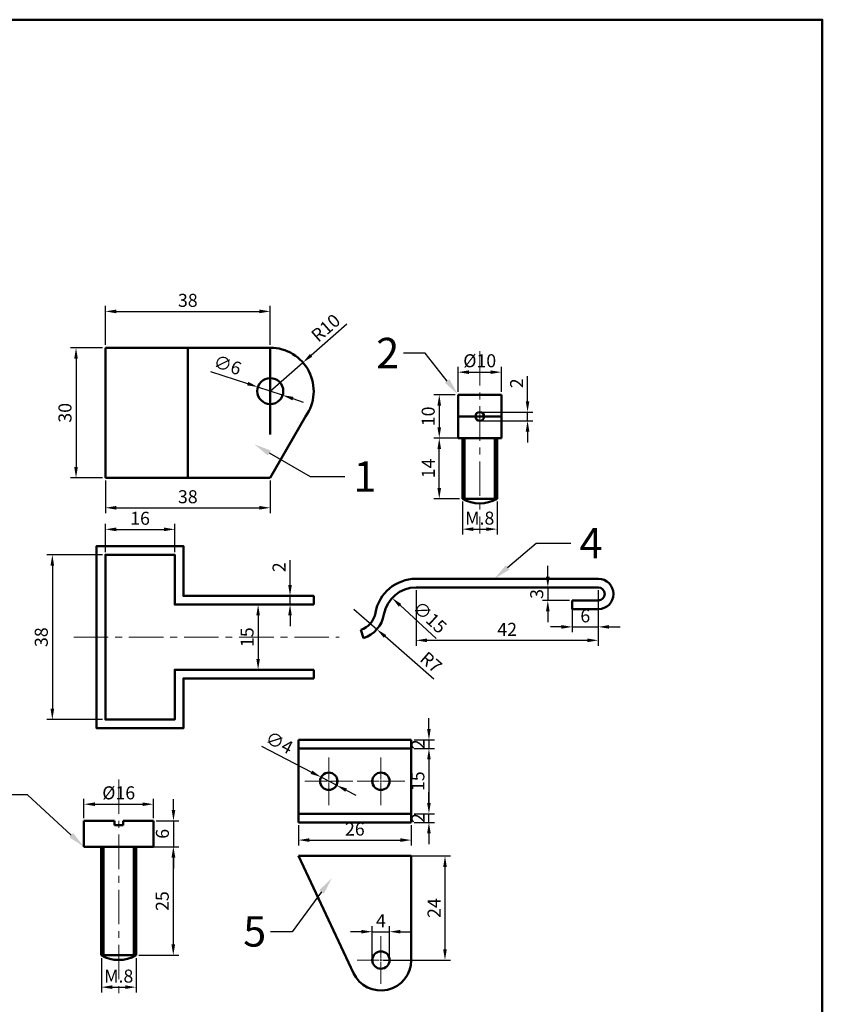
# Model space of a CAD drawing. Units: millimetres. Extents: x 77 to 718, y -35 to 313.
# Tile 7 of 7: x 533 to 718, y 86 to 313. Entities that reach past the tile are written whole.
import ezdxf
from ezdxf import colors
from ezdxf.entities.mleader import LeaderData, LeaderLine
from ezdxf.math import Vec2, Vec3

# ---------------------------------------------------------------- set-up
doc = ezdxf.new("R2010")
doc.units = ezdxf.units.MM
doc.header["$LTSCALE"] = 0.5
doc.linetypes.add('CENTER', pattern=[50.8, 31.75, -6.35, 6.35, -6.35])
for name, color, linetype, lineweight in [('M-CNTR', 1, 'CENTER', 18), ('M-DIMS', 2, 'Continuous', 25), ('M-OUTL', 7, 'Continuous', 50), ('M-TEXT', 3, 'Continuous', 25)]:
    doc.layers.add(name, color=color, linetype=linetype, lineweight=lineweight)
doc.styles.get("Standard").update_dxf_attribs({"font": 'arial.ttf'})
doc.dimstyles.new('ISO-25', dxfattribs={"dimtxt": 3, "dimasz": 2.5, "dimexe": 1.25, "dimexo": 0.625, "dimtad": 1, "dimtxsty": 'Standard', "dimcen": 2.5, "dimadec": 0, "dimazin": 0, "dimtfac": 1, "dimtmove": 0, "dimatfit": 3, "dimfxl": 1, "dimarcsym": 0})

# ---------------------------------------------------------------- blocks, each defined once
blk = doc.blocks.new('*D93')
at = {"layer": 'Defpoints', "color": 0, "ltscale": 0.5, "transparency": 16777216}
for p in [(590.84, 245.68), (552.84, 237.31), (590.84, 237.31)]:
    blk.add_point(p, dxfattribs=at)
at = {"layer": 'M-DIMS', "color": 0, "lineweight": -2, "ltscale": 0.5, "transparency": 16777216}
for p, q in [((552.84, 237.94), (552.84, 246.93)), ((555.34, 245.68), (588.34, 245.68)), ((590.84, 237.94), (590.84, 246.93))]:
    blk.add_line(p, q, dxfattribs=at)
at = {"layer": 'M-DIMS', "color": 0, "ltscale": 0.5, "transparency": 16777216}
for points in [[(555.34, 246.1), (555.34, 245.26), (552.84, 245.68)], [(588.34, 246.1), (588.34, 245.26), (590.84, 245.68)]]:
    blk.add_solid(points, dxfattribs=at)
at = {"layer": 'M-DIMS', "color": 0, "ltscale": 0.5, "transparency": 16777216, "insert": (571.84, 247.84), "char_height": 3, "attachment_point": 5}
blk.add_mtext('38', dxfattribs=at)
blk = doc.blocks.new('*D94')
at = {"layer": 'Defpoints', "color": 0, "ltscale": 0.5, "transparency": 16777216}
for p in [(552.84, 237.31), (546.09, 207.31), (552.84, 207.31)]:
    blk.add_point(p, dxfattribs=at)
at = {"layer": 'M-DIMS', "color": 0, "lineweight": -2, "ltscale": 0.5, "transparency": 16777216}
for p, q in [((552.22, 237.31), (544.84, 237.31)), ((546.09, 234.81), (546.09, 209.81)), ((552.22, 207.31), (544.84, 207.31))]:
    blk.add_line(p, q, dxfattribs=at)
at = {"layer": 'M-DIMS', "color": 0, "ltscale": 0.5, "transparency": 16777216}
for points in [[(545.67, 234.81), (546.5, 234.81), (546.09, 237.31)], [(545.67, 209.81), (546.5, 209.81), (546.09, 207.31)]]:
    blk.add_solid(points, dxfattribs=at)
at = {"layer": 'M-DIMS', "color": 0, "ltscale": 0.5, "transparency": 16777216, "insert": (543.93, 222.31), "char_height": 3, "attachment_point": 5, "rotation": 90}
blk.add_mtext('30', dxfattribs=at)
blk = doc.blocks.new('*D95')
at = {"layer": 'Defpoints', "color": 0, "ltscale": 0.5, "transparency": 16777216}
for p in [(552.84, 207.31), (590.84, 207.31), (590.84, 200.42)]:
    blk.add_point(p, dxfattribs=at)
at = {"layer": 'M-DIMS', "color": 0, "lineweight": -2, "ltscale": 0.5, "transparency": 16777216}
for p, q in [((552.84, 206.69), (552.84, 199.17)), ((590.84, 206.69), (590.84, 199.17)), ((555.34, 200.42), (588.34, 200.42))]:
    blk.add_line(p, q, dxfattribs=at)
at = {"layer": 'M-DIMS', "color": 0, "ltscale": 0.5, "transparency": 16777216}
for points in [[(555.34, 200.84), (555.34, 200.01), (552.84, 200.42)], [(588.34, 200.84), (588.34, 200.01), (590.84, 200.42)]]:
    blk.add_solid(points, dxfattribs=at)
at = {"layer": 'M-DIMS', "color": 0, "ltscale": 0.5, "transparency": 16777216, "insert": (571.84, 202.58), "char_height": 3, "attachment_point": 5}
blk.add_mtext('38', dxfattribs=at)
blk = doc.blocks.new('*D96')
at = {"layer": 'Defpoints', "color": 0, "ltscale": 0.5, "transparency": 16777216}
for p in [(587.99, 228.25), (593.69, 226.37)]:
    blk.add_point(p, dxfattribs=at)
at = {"layer": 'M-DIMS', "color": 0, "lineweight": -2, "ltscale": 0.5, "transparency": 16777216}
for p, q in [((577.1, 231.86), (585.62, 229.04)), ((593.69, 226.37), (587.99, 228.25)), ((596.06, 225.58), (598.44, 224.8))]:
    blk.add_line(p, q, dxfattribs=at)
at = {"layer": 'M-DIMS', "color": 0, "ltscale": 0.5, "transparency": 16777216}
for points in [[(585.75, 229.44), (585.49, 228.64), (587.99, 228.25)], [(596.19, 225.98), (595.93, 225.19), (593.69, 226.37)]]:
    blk.add_solid(points, dxfattribs=at)
at = {"layer": 'M-DIMS', "color": 0, "ltscale": 0.5, "transparency": 16777216, "insert": (580.87, 232.97), "char_height": 3, "attachment_point": 5, "rotation": 341.6845}
blk.add_mtext('∅6', dxfattribs=at)
blk = doc.blocks.new('*D97')
at = {"layer": 'Defpoints', "color": 0, "ltscale": 0.5, "transparency": 16777216}
for p in [(598.36, 233.9), (590.84, 227.31)]:
    blk.add_point(p, dxfattribs=at)
at = {"layer": 'M-DIMS', "color": 0, "lineweight": -2, "ltscale": 0.5, "transparency": 16777216}
for p, q in [((608.44, 242.74), (600.24, 235.55)), ((590.84, 227.31), (598.36, 233.9))]:
    blk.add_line(p, q, dxfattribs=at)
at = {"layer": 'M-DIMS', "color": 0, "ltscale": 0.5, "transparency": 16777216}
blk.add_solid([(599.96, 235.87), (600.51, 235.24), (598.36, 233.9)], dxfattribs=at)
at = {"layer": 'M-DIMS', "color": 0, "ltscale": 0.5, "transparency": 16777216, "insert": (603.86, 241.59), "char_height": 3, "attachment_point": 5, "rotation": 41.2422}
blk.add_mtext('R10', dxfattribs=at)
blk = doc.blocks.new('*D98')
at = {"layer": 'Defpoints', "color": 0, "ltscale": 0.5, "transparency": 16777216}
for p in [(584.84, 178.1), (584.84, 163.1), (588.04, 163.1)]:
    blk.add_point(p, dxfattribs=at)
at = {"layer": 'M-DIMS', "color": 0, "lineweight": -2, "ltscale": 0.5, "transparency": 16777216}
for p, q in [((585.47, 178.1), (589.29, 178.1)), ((588.04, 175.6), (588.04, 165.6)), ((585.47, 163.1), (589.29, 163.1))]:
    blk.add_line(p, q, dxfattribs=at)
at = {"layer": 'M-DIMS', "color": 0, "ltscale": 0.5, "transparency": 16777216}
for points in [[(587.62, 175.6), (588.45, 175.6), (588.04, 178.1)], [(587.62, 165.6), (588.45, 165.6), (588.04, 163.1)]]:
    blk.add_solid(points, dxfattribs=at)
at = {"layer": 'M-DIMS', "color": 0, "ltscale": 0.5, "transparency": 16777216, "insert": (585.88, 170.6), "char_height": 3, "attachment_point": 5, "rotation": 90}
blk.add_mtext('15', dxfattribs=at)
blk = doc.blocks.new('*D99')
at = {"layer": 'Defpoints', "color": 0, "ltscale": 0.5, "transparency": 16777216}
for p in [(568.84, 195.45), (552.84, 189.6), (568.84, 189.6)]:
    blk.add_point(p, dxfattribs=at)
at = {"layer": 'M-DIMS', "color": 0, "lineweight": -2, "ltscale": 0.5, "transparency": 16777216}
for p, q in [((552.84, 190.22), (552.84, 196.7)), ((555.34, 195.45), (566.34, 195.45)), ((568.84, 190.22), (568.84, 196.7))]:
    blk.add_line(p, q, dxfattribs=at)
at = {"layer": 'M-DIMS', "color": 0, "ltscale": 0.5, "transparency": 16777216}
for points in [[(555.34, 195.87), (555.34, 195.03), (552.84, 195.45)], [(566.34, 195.87), (566.34, 195.03), (568.84, 195.45)]]:
    blk.add_solid(points, dxfattribs=at)
at = {"layer": 'M-DIMS', "color": 0, "ltscale": 0.5, "transparency": 16777216, "insert": (560.84, 197.61), "char_height": 3, "attachment_point": 5}
blk.add_mtext('16', dxfattribs=at)
blk = doc.blocks.new('*D100')
at = {"layer": 'Defpoints', "color": 0, "ltscale": 0.5, "transparency": 16777216}
for p in [(552.84, 189.6), (540.63, 151.6), (552.84, 151.6)]:
    blk.add_point(p, dxfattribs=at)
at = {"layer": 'M-DIMS', "color": 0, "lineweight": -2, "ltscale": 0.5, "transparency": 16777216}
for p, q in [((552.22, 189.6), (539.38, 189.6)), ((540.63, 187.1), (540.63, 154.1)), ((552.22, 151.6), (539.38, 151.6))]:
    blk.add_line(p, q, dxfattribs=at)
at = {"layer": 'M-DIMS', "color": 0, "ltscale": 0.5, "transparency": 16777216}
for points in [[(540.21, 187.1), (541.04, 187.1), (540.63, 189.6)], [(540.21, 154.1), (541.04, 154.1), (540.63, 151.6)]]:
    blk.add_solid(points, dxfattribs=at)
at = {"layer": 'M-DIMS', "color": 0, "ltscale": 0.5, "transparency": 16777216, "insert": (538.47, 170.6), "char_height": 3, "attachment_point": 5, "rotation": 90}
blk.add_mtext('38', dxfattribs=at)
blk = doc.blocks.new('*D104')
at = {"layer": 'Defpoints', "color": 0, "ltscale": 0.5, "transparency": 16777216}
for p in [(629.77, 216.49), (635.09, 216.49), (635.09, 202.49)]:
    blk.add_point(p, dxfattribs=at)
at = {"layer": 'M-DIMS', "color": 0, "lineweight": -2, "ltscale": 0.5, "transparency": 16777216}
for p, q in [((634.46, 216.49), (628.52, 216.49)), ((629.77, 204.99), (629.77, 213.99)), ((634.46, 202.49), (628.52, 202.49))]:
    blk.add_line(p, q, dxfattribs=at)
at = {"layer": 'M-DIMS', "color": 0, "ltscale": 0.5, "transparency": 16777216}
for points in [[(629.35, 213.99), (630.18, 213.99), (629.77, 216.49)], [(629.35, 204.99), (630.18, 204.99), (629.77, 202.49)]]:
    blk.add_solid(points, dxfattribs=at)
at = {"layer": 'M-DIMS', "color": 0, "ltscale": 0.5, "transparency": 16777216, "insert": (627.64, 209.49), "char_height": 3, "attachment_point": 5, "rotation": 90}
blk.add_mtext('14', dxfattribs=at)
blk = doc.blocks.new('*D105')
at = {"layer": 'Defpoints', "color": 0, "ltscale": 0.5, "transparency": 16777216}
for p in [(634.09, 226.49), (629.77, 216.49), (634.09, 216.49)]:
    blk.add_point(p, dxfattribs=at)
at = {"layer": 'M-DIMS', "color": 0, "lineweight": -2, "ltscale": 0.5, "transparency": 16777216}
for p, q in [((633.46, 226.49), (628.52, 226.49)), ((629.77, 223.99), (629.77, 218.99)), ((633.46, 216.49), (628.52, 216.49))]:
    blk.add_line(p, q, dxfattribs=at)
at = {"layer": 'M-DIMS', "color": 0, "ltscale": 0.5, "transparency": 16777216}
for points in [[(629.35, 223.99), (630.18, 223.99), (629.77, 226.49)], [(629.35, 218.99), (630.18, 218.99), (629.77, 216.49)]]:
    blk.add_solid(points, dxfattribs=at)
at = {"layer": 'M-DIMS', "color": 0, "ltscale": 0.5, "transparency": 16777216, "insert": (627.61, 221.49), "char_height": 3, "attachment_point": 5, "rotation": 90}
blk.add_mtext('10', dxfattribs=at)
blk = doc.blocks.new('*D106')
at = {"layer": 'Defpoints', "color": 0, "ltscale": 0.5, "transparency": 16777216}
for p in [(644.09, 231.68), (634.09, 226.49), (644.09, 226.49)]:
    blk.add_point(p, dxfattribs=at)
at = {"layer": 'M-DIMS', "color": 0, "lineweight": -2, "ltscale": 0.5, "transparency": 16777216}
for p, q in [((634.09, 227.11), (634.09, 232.93)), ((636.59, 231.68), (641.59, 231.68)), ((644.09, 227.11), (644.09, 232.93))]:
    blk.add_line(p, q, dxfattribs=at)
at = {"layer": 'M-DIMS', "color": 0, "ltscale": 0.5, "transparency": 16777216}
for points in [[(636.59, 232.09), (636.59, 231.26), (634.09, 231.68)], [(641.59, 232.09), (641.59, 231.26), (644.09, 231.68)]]:
    blk.add_solid(points, dxfattribs=at)
at = {"layer": 'M-DIMS', "color": 0, "ltscale": 0.5, "transparency": 16777216, "insert": (639.09, 233.92), "char_height": 3, "attachment_point": 5}
blk.add_mtext('%%C10', dxfattribs=at)
blk = doc.blocks.new('*D107')
at = {"layer": 'Defpoints', "color": 0, "ltscale": 0.5, "transparency": 16777216}
for p in [(639.09, 222.49), (650.11, 222.49), (639.09, 220.49)]:
    blk.add_point(p, dxfattribs=at)
at = {"layer": 'M-DIMS', "color": 0, "lineweight": -2, "ltscale": 0.5, "transparency": 16777216}
for p, q in [((650.11, 224.99), (650.11, 230.72)), ((639.71, 222.49), (651.36, 222.49)), ((650.11, 220.49), (650.11, 222.49)), ((639.71, 220.49), (651.36, 220.49)), ((650.11, 217.99), (650.11, 215.49))]:
    blk.add_line(p, q, dxfattribs=at)
at = {"layer": 'M-DIMS', "color": 0, "ltscale": 0.5, "transparency": 16777216}
for points in [[(649.69, 224.99), (650.53, 224.99), (650.11, 222.49)], [(649.69, 217.99), (650.53, 217.99), (650.11, 220.49)]]:
    blk.add_solid(points, dxfattribs=at)
at = {"layer": 'M-DIMS', "color": 0, "ltscale": 0.5, "transparency": 16777216, "insert": (647.98, 229.11), "char_height": 3, "attachment_point": 5, "rotation": 90}
blk.add_mtext('2', dxfattribs=at)
blk = doc.blocks.new('*D108')
at = {"layer": 'Defpoints', "color": 0, "ltscale": 0.5, "transparency": 16777216}
for p in [(635.09, 202.49), (643.09, 202.49), (643.09, 195.5)]:
    blk.add_point(p, dxfattribs=at)
at = {"layer": 'M-DIMS', "color": 0, "lineweight": -2, "ltscale": 0.5, "transparency": 16777216}
for p, q in [((635.09, 201.86), (635.09, 194.25)), ((643.09, 201.86), (643.09, 194.25)), ((637.59, 195.5), (640.59, 195.5))]:
    blk.add_line(p, q, dxfattribs=at)
at = {"layer": 'M-DIMS', "color": 0, "ltscale": 0.5, "transparency": 16777216}
for points in [[(637.59, 195.91), (637.59, 195.08), (635.09, 195.5)], [(640.59, 195.91), (640.59, 195.08), (643.09, 195.5)]]:
    blk.add_solid(points, dxfattribs=at)
at = {"layer": 'M-DIMS', "color": 0, "ltscale": 0.5, "transparency": 16777216, "insert": (639.09, 197.65), "char_height": 3, "attachment_point": 5}
blk.add_mtext('M.8', dxfattribs=at)
blk = doc.blocks.new('*D109')
at = {"layer": 'Defpoints', "color": 0, "ltscale": 0.5, "transparency": 16777216}
for p in [(563.92, 132.1), (547.92, 128.28), (563.92, 128.28)]:
    blk.add_point(p, dxfattribs=at)
at = {"layer": 'M-DIMS', "color": 0, "lineweight": -2, "ltscale": 0.5, "transparency": 16777216}
for p, q in [((547.92, 128.9), (547.92, 133.35)), ((550.42, 132.1), (561.42, 132.1)), ((563.92, 128.9), (563.92, 133.35))]:
    blk.add_line(p, q, dxfattribs=at)
at = {"layer": 'M-DIMS', "color": 0, "ltscale": 0.5, "transparency": 16777216}
for points in [[(550.42, 132.52), (550.42, 131.69), (547.92, 132.1)], [(561.42, 132.52), (561.42, 131.69), (563.92, 132.1)]]:
    blk.add_solid(points, dxfattribs=at)
at = {"layer": 'M-DIMS', "color": 0, "ltscale": 0.5, "transparency": 16777216, "insert": (555.92, 134.34), "char_height": 3, "attachment_point": 5}
blk.add_mtext('%%C16', dxfattribs=at)
blk = doc.blocks.new('*D110')
at = {"layer": 'Defpoints', "color": 0, "ltscale": 0.5, "transparency": 16777216}
for p in [(563.92, 128.28), (563.84, 122.28), (568.54, 122.28)]:
    blk.add_point(p, dxfattribs=at)
at = {"layer": 'M-DIMS', "color": 0, "lineweight": -2, "ltscale": 0.5, "transparency": 16777216}
for p, q in [((568.54, 130.78), (568.54, 133.28)), ((564.54, 128.28), (569.79, 128.28)), ((568.54, 128.28), (568.54, 122.28)), ((564.46, 122.28), (569.79, 122.28)), ((568.54, 119.78), (568.54, 117.28))]:
    blk.add_line(p, q, dxfattribs=at)
at = {"layer": 'M-DIMS', "color": 0, "ltscale": 0.5, "transparency": 16777216}
for points in [[(568.12, 130.78), (568.96, 130.78), (568.54, 128.28)], [(568.12, 119.78), (568.96, 119.78), (568.54, 122.28)]]:
    blk.add_solid(points, dxfattribs=at)
at = {"layer": 'M-DIMS', "color": 0, "ltscale": 0.5, "transparency": 16777216, "insert": (566.38, 125.28), "char_height": 3, "attachment_point": 5, "rotation": 90}
blk.add_mtext('6', dxfattribs=at)
blk = doc.blocks.new('*D111')
at = {"layer": 'Defpoints', "color": 0, "ltscale": 0.5, "transparency": 16777216}
for p in [(559.92, 122.28), (559.92, 97.28), (568.49, 97.28)]:
    blk.add_point(p, dxfattribs=at)
at = {"layer": 'M-DIMS', "color": 0, "lineweight": -2, "ltscale": 0.5, "transparency": 16777216}
for p, q in [((560.54, 122.28), (569.74, 122.28)), ((568.49, 119.78), (568.49, 99.78)), ((560.54, 97.28), (569.74, 97.28))]:
    blk.add_line(p, q, dxfattribs=at)
at = {"layer": 'M-DIMS', "color": 0, "ltscale": 0.5, "transparency": 16777216}
for points in [[(568.08, 119.78), (568.91, 119.78), (568.49, 122.28)], [(568.08, 99.78), (568.91, 99.78), (568.49, 97.28)]]:
    blk.add_solid(points, dxfattribs=at)
at = {"layer": 'M-DIMS', "color": 0, "ltscale": 0.5, "transparency": 16777216, "insert": (566.34, 109.78), "char_height": 3, "attachment_point": 5, "rotation": 90}
blk.add_mtext('25', dxfattribs=at)
blk = doc.blocks.new('*D112')
at = {"layer": 'Defpoints', "color": 0, "ltscale": 0.5, "transparency": 16777216}
for p in [(551.92, 97.28), (559.92, 97.28), (559.92, 89.94)]:
    blk.add_point(p, dxfattribs=at)
at = {"layer": 'M-DIMS', "color": 0, "lineweight": -2, "ltscale": 0.5, "transparency": 16777216}
for p, q in [((551.92, 96.65), (551.92, 88.69)), ((559.92, 96.65), (559.92, 88.69)), ((554.42, 89.94), (557.42, 89.94))]:
    blk.add_line(p, q, dxfattribs=at)
at = {"layer": 'M-DIMS', "color": 0, "ltscale": 0.5, "transparency": 16777216}
for points in [[(554.42, 90.36), (554.42, 89.53), (551.92, 89.94)], [(557.42, 90.36), (557.42, 89.53), (559.92, 89.94)]]:
    blk.add_solid(points, dxfattribs=at)
at = {"layer": 'M-DIMS', "color": 0, "ltscale": 0.5, "transparency": 16777216, "insert": (555.92, 92.1), "char_height": 3, "attachment_point": 5}
blk.add_mtext('M.8', dxfattribs=at)
blk = doc.blocks.new('*D113')
at = {"layer": 'Defpoints', "color": 0, "ltscale": 0.5, "transparency": 16777216}
for p in [(624.41, 182.06), (666.41, 182.06), (666.41, 169.88)]:
    blk.add_point(p, dxfattribs=at)
at = {"layer": 'M-DIMS', "color": 0, "lineweight": -2, "ltscale": 0.5, "transparency": 16777216}
for p, q in [((624.41, 181.43), (624.41, 168.63)), ((666.41, 181.43), (666.41, 168.63)), ((626.91, 169.88), (663.91, 169.88))]:
    blk.add_line(p, q, dxfattribs=at)
at = {"layer": 'M-DIMS', "color": 0, "ltscale": 0.5, "transparency": 16777216}
for points in [[(626.91, 170.29), (626.91, 169.46), (624.41, 169.88)], [(663.91, 170.29), (663.91, 169.46), (666.41, 169.88)]]:
    blk.add_solid(points, dxfattribs=at)
at = {"layer": 'M-DIMS', "color": 0, "ltscale": 0.5, "transparency": 16777216, "insert": (645.41, 172.01), "char_height": 3, "attachment_point": 5}
blk.add_mtext('42', dxfattribs=at)
blk = doc.blocks.new('*D114')
at = {"layer": 'Defpoints', "color": 0, "ltscale": 0.5, "transparency": 16777216}
for p in [(660.41, 179.06), (666.41, 179.06), (666.41, 172.97)]:
    blk.add_point(p, dxfattribs=at)
at = {"layer": 'M-DIMS', "color": 0, "lineweight": -2, "ltscale": 0.5, "transparency": 16777216}
for p, q in [((660.41, 178.43), (660.41, 171.72)), ((666.41, 178.43), (666.41, 171.72)), ((657.91, 172.97), (655.41, 172.97)), ((660.41, 172.97), (666.41, 172.97)), ((668.91, 172.97), (671.41, 172.97))]:
    blk.add_line(p, q, dxfattribs=at)
at = {"layer": 'M-DIMS', "color": 0, "ltscale": 0.5, "transparency": 16777216}
for points in [[(657.91, 173.39), (657.91, 172.55), (660.41, 172.97)], [(668.91, 173.39), (668.91, 172.55), (666.41, 172.97)]]:
    blk.add_solid(points, dxfattribs=at)
at = {"layer": 'M-DIMS', "color": 0, "ltscale": 0.5, "transparency": 16777216, "insert": (663.41, 175.13), "char_height": 3, "attachment_point": 5}
blk.add_mtext('6', dxfattribs=at)
blk = doc.blocks.new('*D115')
at = {"layer": 'Defpoints', "color": 0, "ltscale": 0.5, "transparency": 16777216}
for p in [(660.41, 182.06), (654.78, 179.06), (660.41, 179.06)]:
    blk.add_point(p, dxfattribs=at)
at = {"layer": 'M-DIMS', "color": 0, "lineweight": -2, "ltscale": 0.5, "transparency": 16777216}
for p, q in [((654.78, 184.56), (654.78, 187.06)), ((659.79, 182.06), (653.53, 182.06)), ((654.78, 182.06), (654.78, 179.06)), ((659.79, 179.06), (653.53, 179.06)), ((654.78, 176.56), (654.78, 174.06))]:
    blk.add_line(p, q, dxfattribs=at)
at = {"layer": 'M-DIMS', "color": 0, "ltscale": 0.5, "transparency": 16777216}
for points in [[(654.36, 184.56), (655.19, 184.56), (654.78, 182.06)], [(654.36, 176.56), (655.19, 176.56), (654.78, 179.06)]]:
    blk.add_solid(points, dxfattribs=at)
at = {"layer": 'M-DIMS', "color": 0, "ltscale": 0.5, "transparency": 16777216, "insert": (652.62, 180.56), "char_height": 3, "attachment_point": 5, "rotation": 90}
blk.add_mtext('3', dxfattribs=at)
blk = doc.blocks.new('*D116')
at = {"layer": 'Defpoints', "color": 0, "ltscale": 0.5, "transparency": 16777216}
for p in [(618.89, 179.64), (629.93, 169.48)]:
    blk.add_point(p, dxfattribs=at)
at = {"layer": 'M-DIMS', "color": 0, "lineweight": -2, "ltscale": 0.5, "transparency": 16777216}
blk.add_line((629.07, 170.27), (620.73, 177.94), dxfattribs=at)
at = {"layer": 'M-DIMS', "color": 0, "ltscale": 0.5, "transparency": 16777216}
blk.add_solid([(621.02, 178.25), (620.45, 177.64), (618.89, 179.64)], dxfattribs=at)
at = {"layer": 'M-DIMS', "color": 0, "ltscale": 0.5, "transparency": 16777216, "insert": (627.34, 174.91), "char_height": 3, "attachment_point": 5, "rotation": 317.367}
blk.add_mtext('∅15', dxfattribs=at)
blk = doc.blocks.new('*D117')
at = {"layer": 'Defpoints', "color": 0, "ltscale": 0.5, "transparency": 16777216}
for p in [(610.12, 177.03), (615.39, 172.42)]:
    blk.add_point(p, dxfattribs=at)
at = {"layer": 'M-DIMS', "color": 0, "lineweight": -2, "ltscale": 0.5, "transparency": 16777216}
for p, q in [((610.12, 177.03), (615.39, 172.42)), ((628.52, 160.93), (617.27, 170.77))]:
    blk.add_line(p, q, dxfattribs=at)
at = {"layer": 'M-DIMS', "color": 0, "ltscale": 0.5, "transparency": 16777216}
blk.add_solid([(617.55, 171.09), (617, 170.46), (615.39, 172.42)], dxfattribs=at)
at = {"layer": 'M-DIMS', "color": 0, "ltscale": 0.5, "transparency": 16777216, "insert": (627.63, 164.53), "char_height": 3, "attachment_point": 5, "rotation": 318.8198}
blk.add_mtext('R7', dxfattribs=at)
blk = doc.blocks.new('*D124')
at = {"layer": 'Defpoints', "color": 0, "ltscale": 0.5, "transparency": 16777216}
for p in [(597.52, 180.1), (595.39, 178.1), (597.52, 178.1)]:
    blk.add_point(p, dxfattribs=at)
at = {"layer": 'M-DIMS', "color": 0, "lineweight": -2, "ltscale": 0.5, "transparency": 16777216}
for p, q in [((595.39, 182.6), (595.39, 188.33)), ((596.89, 180.1), (594.14, 180.1)), ((595.39, 178.1), (595.39, 180.1)), ((596.89, 178.1), (594.14, 178.1)), ((595.39, 175.6), (595.39, 173.1))]:
    blk.add_line(p, q, dxfattribs=at)
at = {"layer": 'M-DIMS', "color": 0, "ltscale": 0.5, "transparency": 16777216}
for points in [[(594.97, 182.6), (595.8, 182.6), (595.39, 180.1)], [(594.97, 175.6), (595.8, 175.6), (595.39, 178.1)]]:
    blk.add_solid(points, dxfattribs=at)
at = {"layer": 'M-DIMS', "color": 0, "ltscale": 0.5, "transparency": 16777216, "insert": (593.25, 186.72), "char_height": 3, "attachment_point": 5, "rotation": 90}
blk.add_mtext('2', dxfattribs=at)
blk = doc.blocks.new('*U127')
at = {"layer": 'M-CNTR', "color": 0, "transparency": 16777216}
for p, q in [((0, 0.4), (0, 5.5)), ((-5.5, 0), (-0.4, 0)), ((0.4, 0), (5.5, 0)), ((0, -5.5), (0, -0.4))]:
    blk.add_line(p, q, dxfattribs=at)
at = {"layer": 'M-CNTR', "color": 0, "linetype": 'Continuous', "transparency": 16777216}
for p, q in [((-0.2, 0), (0.2, 0)), ((0, -0.2), (0, 0.2))]:
    blk.add_line(p, q, dxfattribs=at)
blk = doc.blocks.new('*U128')
at = {"layer": 'M-CNTR', "color": 0, "transparency": 16777216}
for p, q in [((0, 0.4), (0, 5.5)), ((-5.5, 0), (-0.4, 0)), ((0.4, 0), (5.5, 0)), ((0, -5.5), (0, -0.4))]:
    blk.add_line(p, q, dxfattribs=at)
at = {"layer": 'M-CNTR', "color": 0, "linetype": 'Continuous', "transparency": 16777216}
for p, q in [((-0.2, 0), (0.2, 0)), ((0, -0.2), (0, 0.2))]:
    blk.add_line(p, q, dxfattribs=at)
blk = doc.blocks.new('*U129')
at = {"layer": 'M-CNTR', "color": 0, "transparency": 16777216}
for p, q in [((0, 0.4), (0, 5.5)), ((-5.5, 0), (-0.4, 0)), ((0.4, 0), (5.5, 0)), ((0, -5.5), (0, -0.4))]:
    blk.add_line(p, q, dxfattribs=at)
at = {"layer": 'M-CNTR', "color": 0, "linetype": 'Continuous', "transparency": 16777216}
for p, q in [((-0.2, 0), (0.2, 0)), ((0, -0.2), (0, 0.2))]:
    blk.add_line(p, q, dxfattribs=at)
blk = doc.blocks.new('*D130')
at = {"layer": 'Defpoints', "color": 0, "ltscale": 0.5, "transparency": 16777216}
for p in [(623.32, 146.91), (623.32, 144.91), (627.39, 144.91)]:
    blk.add_point(p, dxfattribs=at)
at = {"layer": 'M-DIMS', "color": 0, "lineweight": -2, "ltscale": 0.5, "transparency": 16777216}
for p, q in [((627.39, 149.41), (627.39, 151.91)), ((623.95, 146.91), (628.64, 146.91)), ((627.39, 146.91), (627.39, 144.91)), ((623.95, 144.91), (628.64, 144.91)), ((627.39, 142.41), (627.39, 139.91))]:
    blk.add_line(p, q, dxfattribs=at)
at = {"layer": 'M-DIMS', "color": 0, "ltscale": 0.5, "transparency": 16777216}
for points in [[(626.97, 149.41), (627.8, 149.41), (627.39, 146.91)], [(626.97, 142.41), (627.8, 142.41), (627.39, 144.91)]]:
    blk.add_solid(points, dxfattribs=at)
at = {"layer": 'M-DIMS', "color": 0, "ltscale": 0.5, "transparency": 16777216, "insert": (625.26, 145.91), "char_height": 3, "attachment_point": 5, "rotation": 90}
blk.add_mtext('2', dxfattribs=at)
blk = doc.blocks.new('*D131')
at = {"layer": 'Defpoints', "color": 0, "ltscale": 0.5, "transparency": 16777216}
for p in [(623.32, 144.91), (623.32, 129.91), (627.39, 129.91)]:
    blk.add_point(p, dxfattribs=at)
at = {"layer": 'M-DIMS', "color": 0, "lineweight": -2, "ltscale": 0.5, "transparency": 16777216}
for p, q in [((623.95, 144.91), (628.64, 144.91)), ((627.39, 142.41), (627.39, 132.41)), ((623.95, 129.91), (628.64, 129.91))]:
    blk.add_line(p, q, dxfattribs=at)
at = {"layer": 'M-DIMS', "color": 0, "ltscale": 0.5, "transparency": 16777216}
for points in [[(626.97, 142.41), (627.8, 142.41), (627.39, 144.91)], [(626.97, 132.41), (627.8, 132.41), (627.39, 129.91)]]:
    blk.add_solid(points, dxfattribs=at)
at = {"layer": 'M-DIMS', "color": 0, "ltscale": 0.5, "transparency": 16777216, "insert": (625.23, 137.41), "char_height": 3, "attachment_point": 5, "rotation": 90}
blk.add_mtext('15', dxfattribs=at)
blk = doc.blocks.new('*D132')
at = {"layer": 'Defpoints', "color": 0, "ltscale": 0.5, "transparency": 16777216}
for p in [(623.32, 129.91), (627.39, 129.91), (623.32, 127.91)]:
    blk.add_point(p, dxfattribs=at)
at = {"layer": 'M-DIMS', "color": 0, "lineweight": -2, "ltscale": 0.5, "transparency": 16777216}
for p, q in [((627.39, 132.41), (627.39, 134.91)), ((623.95, 129.91), (628.64, 129.91)), ((627.39, 127.91), (627.39, 129.91)), ((623.95, 127.91), (628.64, 127.91)), ((627.39, 125.41), (627.39, 122.91))]:
    blk.add_line(p, q, dxfattribs=at)
at = {"layer": 'M-DIMS', "color": 0, "ltscale": 0.5, "transparency": 16777216}
for points in [[(626.97, 132.41), (627.8, 132.41), (627.39, 129.91)], [(626.97, 125.41), (627.8, 125.41), (627.39, 127.91)]]:
    blk.add_solid(points, dxfattribs=at)
at = {"layer": 'M-DIMS', "color": 0, "ltscale": 0.5, "transparency": 16777216, "insert": (625.26, 128.91), "char_height": 3, "attachment_point": 5, "rotation": 90}
blk.add_mtext('2', dxfattribs=at)
blk = doc.blocks.new('*D133')
at = {"layer": 'Defpoints', "color": 0, "ltscale": 0.5, "transparency": 16777216}
for p in [(597.32, 127.91), (623.32, 127.91), (623.32, 123.84)]:
    blk.add_point(p, dxfattribs=at)
at = {"layer": 'M-DIMS', "color": 0, "lineweight": -2, "ltscale": 0.5, "transparency": 16777216}
for p, q in [((597.32, 127.28), (597.32, 122.59)), ((623.32, 127.28), (623.32, 122.59)), ((599.82, 123.84), (620.82, 123.84))]:
    blk.add_line(p, q, dxfattribs=at)
at = {"layer": 'M-DIMS', "color": 0, "ltscale": 0.5, "transparency": 16777216}
for points in [[(599.82, 124.25), (599.82, 123.42), (597.32, 123.84)], [(620.82, 124.25), (620.82, 123.42), (623.32, 123.84)]]:
    blk.add_solid(points, dxfattribs=at)
at = {"layer": 'M-DIMS', "color": 0, "ltscale": 0.5, "transparency": 16777216, "insert": (610.32, 125.99), "char_height": 3, "attachment_point": 5}
blk.add_mtext('26', dxfattribs=at)
blk = doc.blocks.new('*D134')
at = {"layer": 'Defpoints', "color": 0, "ltscale": 0.5, "transparency": 16777216}
for p in [(616.32, 120.17), (616.32, 96.17), (631.09, 96.17)]:
    blk.add_point(p, dxfattribs=at)
at = {"layer": 'M-DIMS', "color": 0, "lineweight": -2, "ltscale": 0.5, "transparency": 16777216}
for p, q in [((616.95, 120.17), (632.34, 120.17)), ((631.09, 117.67), (631.09, 98.67)), ((616.95, 96.17), (632.34, 96.17))]:
    blk.add_line(p, q, dxfattribs=at)
at = {"layer": 'M-DIMS', "color": 0, "ltscale": 0.5, "transparency": 16777216}
for points in [[(630.67, 117.67), (631.5, 117.67), (631.09, 120.17)], [(630.67, 98.67), (631.5, 98.67), (631.09, 96.17)]]:
    blk.add_solid(points, dxfattribs=at)
at = {"layer": 'M-DIMS', "color": 0, "ltscale": 0.5, "transparency": 16777216, "insert": (628.96, 108.17), "char_height": 3, "attachment_point": 5, "rotation": 90}
blk.add_mtext('24', dxfattribs=at)
blk = doc.blocks.new('*D135')
at = {"layer": 'Defpoints', "color": 0, "ltscale": 0.5, "transparency": 16777216}
for p in [(602.55, 138.33), (606.1, 136.48)]:
    blk.add_point(p, dxfattribs=at)
at = {"layer": 'M-DIMS', "color": 0, "lineweight": -2, "ltscale": 0.5, "transparency": 16777216}
for p, q in [((588.83, 145.47), (600.33, 139.48)), ((606.1, 136.48), (602.55, 138.33)), ((608.31, 135.33), (610.53, 134.17))]:
    blk.add_line(p, q, dxfattribs=at)
at = {"layer": 'M-DIMS', "color": 0, "ltscale": 0.5, "transparency": 16777216}
for points in [[(600.52, 139.85), (600.14, 139.11), (602.55, 138.33)], [(608.51, 135.7), (608.12, 134.96), (606.1, 136.48)]]:
    blk.add_solid(points, dxfattribs=at)
at = {"layer": 'M-DIMS', "color": 0, "ltscale": 0.5, "transparency": 16777216, "insert": (592.74, 145.96), "char_height": 3, "attachment_point": 5, "rotation": 332.5001}
blk.add_mtext('∅4', dxfattribs=at)
blk = doc.blocks.new('*D136')
at = {"layer": 'Defpoints', "color": 0, "ltscale": 0.5, "transparency": 16777216}
for p in [(618.32, 102.72), (614.32, 96.17), (618.32, 96.17)]:
    blk.add_point(p, dxfattribs=at)
at = {"layer": 'M-DIMS', "color": 0, "lineweight": -2, "ltscale": 0.5, "transparency": 16777216}
for p, q in [((611.82, 102.72), (609.32, 102.72)), ((614.32, 96.79), (614.32, 103.97)), ((614.32, 102.72), (618.32, 102.72)), ((618.32, 96.79), (618.32, 103.97)), ((620.82, 102.72), (623.32, 102.72))]:
    blk.add_line(p, q, dxfattribs=at)
at = {"layer": 'M-DIMS', "color": 0, "ltscale": 0.5, "transparency": 16777216}
for points in [[(611.82, 103.14), (611.82, 102.31), (614.32, 102.72)], [(620.82, 103.14), (620.82, 102.31), (618.32, 102.72)]]:
    blk.add_solid(points, dxfattribs=at)
at = {"layer": 'M-DIMS', "color": 0, "ltscale": 0.5, "transparency": 16777216, "insert": (616.32, 104.85), "char_height": 3, "attachment_point": 5}
blk.add_mtext('4', dxfattribs=at)
blk = doc.blocks.new('BRACKET-PLATE')
at = {"ltscale": 0.5}
for p, q in [((0, 31), (26, 31)), ((12.66, 4.03), (0, 31)), ((26, 31), (26, 7))]:
    blk.add_line(p, q, dxfattribs=at)
blk.add_arc((19, 7), 7, 205.1481, 0, dxfattribs=at)

msp = doc.modelspace()

# ---------------------------------------------------------------- linework, layer by layer
at = {"layer": 'M-CNTR', "ltscale": 0.5}
for p, q in [((639.088, 236.509), (639.088, 194.501)), ((545.584, 170.597), (606.698, 170.597)), ((555.916, 137.797), (555.916, 87.326))]:
    msp.add_line(p, q, dxfattribs=at)
at = {"layer": 'M-OUTL', "ltscale": 0.5}
for p, q in [((552.84, 237.312), (590.84, 237.312)), ((552.84, 207.312), (552.84, 237.312)), ((571.84, 207.312), (571.84, 237.312)), ((590.84, 237.312), (590.84, 217.312)), ((634.088, 226.488), (644.088, 226.488)), ((634.088, 216.488), (634.088, 226.488)), ((644.088, 226.488), (644.088, 216.488)), ((598.965, 221.482), (590.84, 207.312)), ((634.088, 221.488), (644.088, 221.488)), ((644.088, 216.488), (634.088, 216.488)), ((635.088, 202.488), (635.088, 216.488)), ((635.588, 202.488), (635.588, 216.488)), ((642.588, 202.488), (642.588, 216.488)), ((643.088, 202.488), (643.088, 216.488)), ((590.84, 207.312), (552.84, 207.312)), ((639.088, 202.488), (635.088, 202.488)), ((639.088, 202.488), (643.088, 202.488)), ((600.84, 180.097), (600.84, 178.097)), ((660.411, 179.055), (660.411, 177.055)), ((611.689, 172.279), (612.316, 170.379)), ((600.84, 163.097), (600.84, 161.097)), ((597.323, 146.906), (597.323, 127.906)), ((623.323, 146.906), (597.323, 146.906)), ((623.323, 127.906), (623.323, 146.906)), ((623.323, 144.906), (597.323, 144.906)), ((597.323, 129.906), (623.323, 129.906)), ((547.915, 128.279), (554.915, 128.279)), ((547.915, 128.279), (547.915, 122.279)), ((554.915, 128.279), (554.915, 127.279)), ((554.915, 127.279), (555.915, 127.279)), ((555.915, 127.279), (556.915, 127.279)), ((556.915, 127.279), (556.915, 128.279)), ((556.915, 128.279), (563.915, 128.279)), ((563.915, 128.279), (563.915, 122.279)), ((597.323, 127.906), (623.323, 127.906)), ((547.915, 122.279), (563.915, 122.279)), ((551.915, 97.279), (551.917, 122.279)), ((552.415, 97.279), (552.415, 122.279)), ((559.415, 97.279), (559.415, 122.279)), ((559.915, 97.279), (559.915, 122.279)), ((555.915, 97.279), (551.915, 97.279)), ((555.915, 97.279), (559.915, 97.279))]:
    msp.add_line(p, q, dxfattribs=at)
msp.add_lwpolyline([(77.418, 312.912), (718.012, 312.912), (718.012, -34.898), (77.418, -34.898)], close=True, dxfattribs=at)
for points in [[(600.84, 161.097), (570.84, 161.097), (570.84, 149.597), (550.84, 149.597), (550.84, 191.597), (570.84, 191.597), (570.84, 180.097), (600.84, 180.097)], [(600.84, 163.097), (568.84, 163.097), (568.84, 151.597), (552.84, 151.597), (552.84, 189.597), (568.84, 189.597), (568.84, 178.097), (600.84, 178.097)]]:
    msp.add_lwpolyline(points, dxfattribs=at)
for points in [[(611.689, 172.279, 0.2770282), (615.051, 176.175, -0.3648802), (624.411, 184.055), (666.411, 184.055, -1), (666.411, 177.055), (660.411, 177.055)], [(612.316, 170.379, 0.2770282), (617.021, 175.834, -0.3648802), (624.411, 182.055), (666.411, 182.055, -1), (666.411, 179.055), (660.411, 179.055)]]:
    msp.add_lwpolyline(points, format="xyb", dxfattribs=at)
for centre, radius in [((590.84, 227.312), 3), ((639.088, 221.488), 1), ((604.323, 137.406), 2), ((616.323, 137.406), 2), ((616.323, 96.17), 2)]:
    msp.add_circle(centre, radius, dxfattribs=at)
for centre, radius, start, end in [((590.84, 227.312), 10, 324.34264, 90), ((639.088, 209.416), 8, 240, 300), ((555.915, 104.207), 8, 239.99853, 299.99853)]:
    msp.add_arc(centre, radius, start, end, dxfattribs=at)

# ---------------------------------------------------------------- block references
at = {"layer": 'M-CNTR'}
for name, p in [('*U129', (604.323, 137.406)), ('*U128', (616.323, 137.406)), ('*U127', (616.323, 96.17))]:
    msp.add_blockref(name, p, dxfattribs=at)
at = {"layer": 'M-OUTL'}
msp.add_blockref('BRACKET-PLATE', (597.323, 89.169), dxfattribs=at)

# ---------------------------------------------------------------- dimensions: what is measured, and where the dimension line sits
at = {"layer": 'M-DIMS', "ltscale": 0.5}
for base, p1, p2, picture, middle in [((590.84, 245.681), (552.84, 237.312), (590.84, 237.312), '*D93', (571.84, 247.839)), ((590.84, 200.424), (552.84, 207.312), (590.84, 207.312), '*D95', (571.84, 202.582)), ((568.84, 195.45), (552.84, 189.597), (568.84, 189.597), '*D99', (560.84, 197.606)), ((666.411, 169.876), (624.411, 182.055), (666.411, 182.055), '*D113', (645.411, 172.007)), ((666.411, 172.972), (660.411, 179.055), (666.411, 179.055), '*D114', (663.411, 175.128)), ((623.323, 123.838), (597.323, 127.906), (623.323, 127.906), '*D133', (610.323, 125.995)), ((618.323, 102.724), (614.323, 96.17), (618.323, 96.17), '*D136', (616.323, 104.849))]:
    dim = msp.add_linear_dim(base=base, p1=p1, p2=p2, dimstyle='ISO-25', override={"dimclrd": 0, "dimclre": 0, "dimclrt": 0}, dxfattribs=at)
    dim.commit()
    dim.dimension.update_dxf_attribs({"geometry": picture, "text_midpoint": middle})
dim = msp.add_radius_dim(center=(590.84, 227.312), mpoint=(598.36, 233.904), dimstyle='ISO-25', override={"dimclrd": 0, "dimclre": 0, "dimclrt": 0}, dxfattribs=at)
dim.commit()
dim.dimension.update_dxf_attribs({"geometry": '*D97', "text_midpoint": (603.859, 241.593)})
for base, p1, p2, picture, middle in [((546.085, 207.312), (552.84, 237.312), (552.84, 207.312), '*D94', (543.928, 222.312)), ((650.111, 222.488), (639.088, 220.488), (639.088, 222.488), '*D107', (647.98, 229.106)), ((629.768, 216.488), (634.088, 226.488), (634.088, 216.488), '*D105', (627.611, 221.488)), ((629.768, 216.488), (635.088, 202.488), (635.088, 216.488), '*D104', (627.637, 209.488)), ((540.625, 151.597), (552.84, 189.597), (552.84, 151.597), '*D100', (538.467, 170.597)), ((588.035, 163.097), (584.84, 178.097), (584.84, 163.097), '*D98', (585.879, 170.597)), ((627.386, 129.906), (623.323, 144.906), (623.323, 129.906), '*D131', (625.23, 137.406)), ((568.541, 122.28), (563.915, 128.279), (563.839, 122.28), '*D110', (566.384, 125.279)), ((568.492, 97.279), (559.915, 122.279), (559.915, 97.279), '*D111', (566.335, 109.779)), ((631.088, 96.17), (616.323, 120.17), (616.323, 96.17), '*D134', (628.957, 108.17))]:
    dim = msp.add_linear_dim(base=base, p1=p1, p2=p2, angle=90, dimstyle='ISO-25', override={"dimclrd": 0, "dimclre": 0, "dimclrt": 0}, dxfattribs=at)
    dim.commit()
    dim.dimension.update_dxf_attribs({"geometry": picture, "text_midpoint": middle})
dim = msp.add_diameter_dim_2p(p1=(593.688, 226.369), p2=(587.992, 228.254), dimstyle='ISO-25', override={"dimclrd": 0, "dimclre": 0, "dimclrt": 0}, dxfattribs=at)
dim.commit()
dim.dimension.update_dxf_attribs({"geometry": '*D96', "text_midpoint": (580.875, 232.971)})
for base, p1, p2, text, picture, middle in [((644.088, 231.676), (634.088, 226.488), (644.088, 226.488), '%%C<>', '*D106', (639.088, 233.916)), ((643.088, 195.496), (635.088, 202.488), (643.088, 202.488), 'M.<>', '*D108', (639.088, 197.653)), ((563.915, 132.104), (547.915, 128.279), (563.915, 128.279), '%%C<>', '*D109', (555.915, 134.345)), ((559.915, 89.943), (551.915, 97.279), (559.915, 97.279), 'M.<>', '*D112', (555.915, 92.099))]:
    dim = msp.add_linear_dim(base=base, p1=p1, p2=p2, text=text, dimstyle='ISO-25', override={"dimclrd": 0, "dimclre": 0, "dimclrt": 0}, dxfattribs=at)
    dim.commit()
    dim.dimension.update_dxf_attribs({"geometry": picture, "text_midpoint": middle})
for base, p1, p2, picture, middle in [((595.386, 178.097), (597.517, 180.097), (597.517, 178.097), '*D124', (595.386, 186.716)), ((654.777, 179.055), (660.411, 182.055), (660.411, 179.055), '*D115', (654.777, 180.555)), ((627.386, 144.906), (623.323, 146.906), (623.323, 144.906), '*D130', (627.386, 145.906)), ((627.386, 129.906), (623.323, 127.906), (623.323, 129.906), '*D132', (627.386, 128.906))]:
    dim = msp.add_linear_dim(base=base, p1=p1, p2=p2, angle=90, dimstyle='ISO-25', override={"dimclrd": 0, "dimclre": 0, "dimclrt": 0}, dxfattribs=at)
    dim.commit()
    dim.dimension.update_dxf_attribs({"geometry": picture, "text_midpoint": middle, "dimtype": 160})
for p1, p2, picture, middle in [((629.929, 169.476), (618.894, 179.635), '*D116', (625.822, 173.257)), ((606.097, 136.483), (602.549, 138.33), '*D135', (591.7, 143.977))]:
    dim = msp.add_diameter_dim_2p(p1=p1, p2=p2, dimstyle='ISO-25', override={"dimclrd": 0, "dimclre": 0, "dimclrt": 0}, dxfattribs=at)
    dim.commit()
    dim.dimension.update_dxf_attribs({"geometry": picture, "text_midpoint": middle, "dimtype": 163})
dim = msp.add_radius_dim(center=(610.124, 177.027), mpoint=(615.392, 172.418), dimstyle='ISO-25', override={"dimclrd": 0, "dimclre": 0, "dimclrt": 0}, dxfattribs=at)
dim.commit()
dim.dimension.update_dxf_attribs({"geometry": '*D117', "text_midpoint": (626.233, 162.935), "dimtype": 164})

# ---------------------------------------------------------------- leaders
at = {"layer": 'M-TEXT', "ltscale": 0.5}
ml = msp.add_multileader_mtext('Standard', dxfattribs=at)
ml.set_content('2', color=256)
ml.set_leader_properties()
ml.build(insert=Vec2(0, 0))
ml.multileader.update_dxf_attribs({"dogleg_length": 5})
ctx = ml.context
ctx.base_point, ctx.char_height, ctx.landing_gap_size, ctx.plane_origin = Vec3(614.909, 236.087), 7, 1, Vec3(634.088, 226.488)
ctx.text_align_type = 2
notes = []
notes.append((ctx, [(0, (1, 1, 0), (626.545, 236.087), (-1, 0), 5, [(0, [(634.088, 226.488)], 0, [])])]))
ctx.mtext.insert, ctx.mtext.alignment, ctx.mtext.flow_direction = Vec3(620.545, 239.587), 3, 5
ml = msp.add_multileader_mtext('Standard', dxfattribs=at)
ml.set_content('1', color=256)
ml.set_leader_properties()
ml.build(insert=Vec2(0, 0))
ctx = ml.context
ctx.base_point, ctx.char_height, ctx.plane_origin = Vec3(608.011, 207.627), 7, Vec3(587.152, 215.051)
notes.append((ctx, [(0, (1, 1, 0), (600.011, 207.627), (1, 0), 8, [(0, [(587.152, 215.051)], 0, [])])]))
ctx.mtext.insert, ctx.mtext.flow_direction = Vec3(610.011, 211.127), 5
ml = msp.add_multileader_mtext('Standard', dxfattribs=at)
ml.set_content('4', color=256)
ml.set_leader_properties()
ml.build(insert=Vec2(0, 0))
ctx = ml.context
ctx.base_point, ctx.char_height, ctx.plane_origin = Vec3(660.075, 192.28), 7, Vec3(642.469, 184.055)
notes.append((ctx, [(0, (1, 1, 0), (652.075, 192.28), (1, 0), 8, [(0, [(642.469, 184.055)], 0, [])])]))
ctx.mtext.insert, ctx.mtext.flow_direction = Vec3(662.075, 195.78), 5
ml = msp.add_multileader_mtext('Standard', dxfattribs=at)
ml.set_content('7', color=256)
ml.set_leader_properties()
ml.build(insert=Vec2(0, 0))
ctx = ml.context
ctx.base_point, ctx.char_height, ctx.plane_origin = Vec3(518.358, 134.277), 7, Vec3(547.915, 122.279)
ctx.text_align_type = 2
notes.append((ctx, [(0, (1, 1, 0), (534.889, 134.277), (-1, 0), 8, [(0, [(547.915, 122.279)], 0, [])])]))
ctx.mtext.insert, ctx.mtext.alignment, ctx.mtext.flow_direction = Vec3(524.889, 137.777), 3, 5
ml = msp.add_multileader_mtext('Standard', dxfattribs=at)
ml.set_content('5', color=256)
ml.set_leader_properties()
ml.build(insert=Vec2(0, 0))
ml.multileader.update_dxf_attribs({"dogleg_length": 5})
ctx = ml.context
ctx.base_point, ctx.char_height, ctx.landing_gap_size, ctx.plane_origin = Vec3(584.256, 102.729), 7, 1, Vec3(605.037, 115.096)
ctx.text_align_type = 2
notes.append((ctx, [(0, (1, 1, 0), (595.897, 102.729), (-1, 0), 5, [(0, [(605.037, 115.096)], 0, [])])]))
ctx.mtext.insert, ctx.mtext.alignment, ctx.mtext.flow_direction = Vec3(589.897, 106.289), 3, 5
for ctx, leaders in notes:
    for number, flags, end, landing, length, lines in leaders:
        leader = LeaderData()
        leader.index, (leader.has_last_leader_line, leader.has_dogleg_vector, leader.attachment_direction) = number, flags
        leader.last_leader_point, leader.dogleg_vector, leader.dogleg_length = Vec3(end), Vec3(landing), length
        for number, points, colour, breaks in lines:
            line = LeaderLine()
            line.index, line.vertices, line.color, line.breaks = number, Vec3.list(points), colors.encode_raw_color(colour), breaks
            leader.lines.append(line)
        ctx.leaders.append(leader)

doc.saveas('drawing.dxf')
